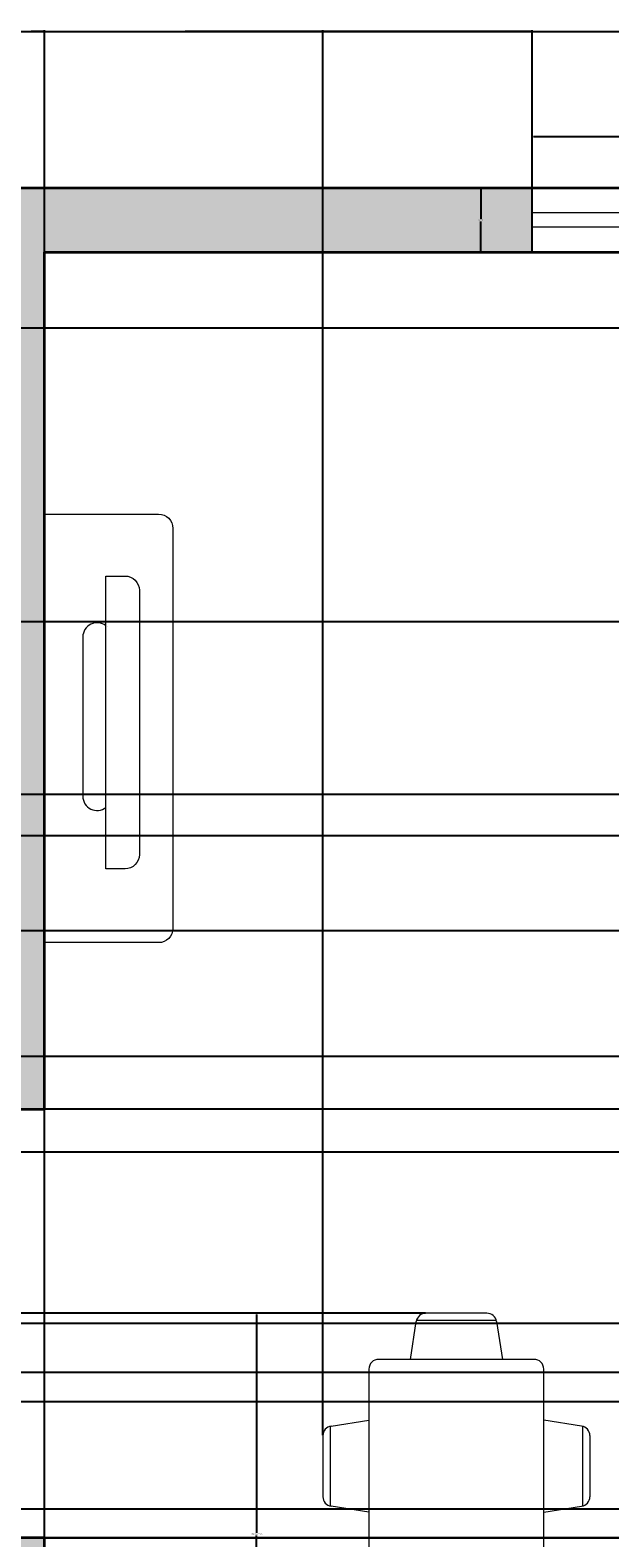
# Model space of a CAD drawing. Units: inches. Extents: x 2800 to 3283, y 1752 to 2114.
# Tile 4 of 6: x 2954 to 3035, y 1903 to 2114. Entities that reach past the tile are written whole.
import ezdxf

# ---------------------------------------------------------------- set-up
doc = ezdxf.new("R2010")
doc.units = ezdxf.units.IN
for name, color, linetype, lineweight in [('A-ANNO-DIMS', 2, 'Continuous', 18), ('A-FURN', 9, 'Continuous', 18), ('A-GLAZ', 4, 'Continuous', 18), ('A-WALL', 7, 'Continuous', 35)]:
    doc.layers.add(name, color=color, linetype=linetype, lineweight=lineweight)
doc.layers.add('A-WALL-PATT', color=18, linetype='Continuous', lineweight=13, true_color=0x000000)
doc.styles.get("Standard").update_dxf_attribs({"font": 'arial.ttf'})
doc.dimstyles.get("Standard").update_dxf_attribs({"dimtxt": 0.18, "dimasz": 0.18, "dimexe": 0.18, "dimexo": 0.0625, "dimgap": 0.09, "dimtad": 0, "dimtih": 1, "dimtoh": 1, "dimdec": 4, "dimzin": 0, "dimdsep": 46, "dimtxsty": 'Standard', "dimcen": 0.09, "dimadec": 0, "dimazin": 0, "dimtfac": 1, "dimtdec": 4, "dimtofl": 0, "dimtmove": 0, "dimatfit": 3, "dimfxl": 1, "dimtolj": 1, "dimtzin": 0, "dimarcsym": 0})

# ---------------------------------------------------------------- blocks, each defined once
blk = doc.blocks.new('Dining Set - 36 x 72 in.')
for p, q in [((-22.26, 25.81), (-23.48, 18)), ((-22.22, 26), (-5.78, 26)), ((-20.29, 27.5), (-7.71, 27.5)), ((-4.52, 18), (-5.74, 25.81)), ((5.74, 25.81), (4.52, 18)), ((5.78, 26), (22.22, 26)), ((7.71, 27.5), (20.29, 27.5)), ((23.48, 18), (22.26, 25.81)), ((-36, 16), (-36, -16)), ((34, 18), (-34, 18)), ((36, -16), (36, 16)), ((-43.81, 8.26), (-36, 9.48)), ((43.81, 8.26), (36, 9.48)), ((-45.5, 6.29), (-45.5, -6.29)), ((-44, 8.22), (-44, -8.22)), ((44, 8.22), (44, -8.22)), ((45.5, 6.29), (45.5, -6.29)), ((-36, -9.48), (-43.81, -8.26)), ((36, -9.48), (43.81, -8.26)), ((-34, -18), (34, -18)), ((-22.26, -25.81), (-23.48, -18)), ((-4.52, -18), (-5.74, -25.81)), ((5.74, -25.81), (4.52, -18)), ((23.48, -18), (22.26, -25.81)), ((-22.22, -26), (-5.78, -26)), ((-20.29, -27.5), (-7.71, -27.5)), ((5.78, -26), (22.22, -26)), ((7.71, -27.5), (20.29, -27.5))]:
    blk.add_line(p, q)
for centre, start, end in [((-20.29, 25.5), 90, 171.1198), ((-7.71, 25.5), 8.881, 90), ((7.71, 25.5), 90, 171.1198), ((20.29, 25.5), 8.881, 90), ((-34, 16), 90, 180), ((34, 16), 0, 90), ((-43.5, 6.29), 98.8806, 180), ((43.5, 6.29), 0, 81.1194), ((-43.5, -6.29), 180, 261.1194), ((43.5, -6.29), 278.8806, 0), ((-34, -16), 180, 270), ((34, -16), 270, 0), ((-20.29, -25.5), 188.8802, 270), ((-7.71, -25.5), 270, 351.1191), ((7.71, -25.5), 188.8802, 270), ((20.29, -25.5), 270, 351.1191)]:
    blk.add_arc(centre, 2, start, end)
blk = doc.blocks.new('WIN-48')
for p, q in [((0, 5.5), (48, 5.5)), ((0, 3.5), (48, 3.5))]:
    blk.add_line(p, q)
for points in [[(0, 0), (0, 9)], [(48, 9), (48, 0)]]:
    blk.add_lwpolyline(points)
blk = doc.blocks.new('MEDIA-CONSOLE-60')
for points in [[(0, 60), (16, 60, -0.414214), (18, 58), (18, 2, -0.414214), (16, 0), (0, 0)], [(8.61, 51.33), (11.3, 51.33, -0.414214), (13.3, 49.33), (13.3, 12.33, -0.414214), (11.3, 10.33), (8.61, 10.33)]]:
    blk.add_lwpolyline(points, format="xyb", close=True)
blk.add_lwpolyline([(8.61, 15.1), (8.61, 47.68)])
blk.add_lwpolyline([(8.61, 44.37, 0.62446), (5.38, 42.79), (5.38, 20.5, 0.62446), (8.61, 18.92, 0.62446)], format="xyb")
blk = doc.blocks.new('*D19')
at = {"layer": 'A-ANNO-DIMS', "color": 0, "lineweight": -2, "transparency": 16777216}
for p, q in [((3023.88, 2092.33), (3023.88, 2099.65)), ((3024.06, 2099.47), (3046.76, 2099.47)), ((3071.7, 2099.47), (3049, 2099.47)), ((3071.88, 2092.33), (3071.88, 2099.65))]:
    blk.add_line(p, q, dxfattribs=at)
at = {"layer": 'A-ANNO-DIMS', "color": 0, "transparency": 16777216}
for points in [[(3024.06, 2099.5), (3024.06, 2099.44), (3023.88, 2099.47)], [(3071.7, 2099.5), (3071.7, 2099.44), (3071.88, 2099.47)]]:
    blk.add_solid(points, dxfattribs=at)
at = {"layer": 'Defpoints', "color": 0, "transparency": 16777216}
for p in [(3023.88, 2099.47), (3023.88, 2092.27), (3071.88, 2092.27)]:
    blk.add_point(p, dxfattribs=at)
at = {"layer": 'A-ANNO-DIMS', "color": 0, "transparency": 16777216, "insert": (3047.88, 2099.47), "char_height": 0.18, "attachment_point": 5}
blk.add_mtext('\\A1;WINDOW 48 TYP.', dxfattribs=at)
blk = doc.blocks.new('*D20')
at = {"layer": 'A-ANNO-DIMS', "color": 0, "lineweight": -2, "transparency": 16777216}
for p, q in [((3023.82, 2092.27), (3016.5, 2092.27)), ((3016.68, 2092.09), (3016.68, 2087.95)), ((3016.68, 2083.45), (3016.68, 2087.59)), ((3023.82, 2083.27), (3016.5, 2083.27))]:
    blk.add_line(p, q, dxfattribs=at)
at = {"layer": 'A-ANNO-DIMS', "color": 0, "transparency": 16777216}
for points in [[(3016.65, 2092.09), (3016.71, 2092.09), (3016.68, 2092.27)], [(3016.65, 2083.45), (3016.71, 2083.45), (3016.68, 2083.27)]]:
    blk.add_solid(points, dxfattribs=at)
at = {"layer": 'Defpoints', "color": 0, "transparency": 16777216}
for p in [(3023.88, 2092.27), (3016.68, 2083.27), (3023.88, 2083.27)]:
    blk.add_point(p, dxfattribs=at)
at = {"layer": 'A-ANNO-DIMS', "color": 0, "transparency": 16777216, "insert": (3016.68, 2087.77), "char_height": 0.18, "attachment_point": 5}
blk.add_mtext('\\A1;9 TYP.', dxfattribs=at)
blk = doc.blocks.new('*D35')
at = {"layer": 'A-ANNO-DIMS', "color": 0, "lineweight": -2, "transparency": 16777216}
for p, q in [((2994.48, 1934.72), (2985.08, 1934.72)), ((2985.26, 1934.54), (2985.26, 1903.97)), ((2985.26, 1873.03), (2985.26, 1903.6)), ((2994.48, 1872.85), (2985.08, 1872.85))]:
    blk.add_line(p, q, dxfattribs=at)
at = {"layer": 'A-ANNO-DIMS', "color": 0, "transparency": 16777216}
for points in [[(2985.23, 1934.54), (2985.29, 1934.54), (2985.26, 1934.72)], [(2985.23, 1873.03), (2985.29, 1873.03), (2985.26, 1872.85)]]:
    blk.add_solid(points, dxfattribs=at)
at = {"layer": 'Defpoints', "color": 0, "transparency": 16777216}
for p in [(2994.54, 1934.72), (2985.26, 1872.85), (2994.54, 1872.85)]:
    blk.add_point(p, dxfattribs=at)
at = {"layer": 'A-ANNO-DIMS', "color": 0, "transparency": 16777216, "insert": (2985.26, 1903.79), "char_height": 0.18, "attachment_point": 5}
blk.add_mtext('\\A1;DINING SET 62', dxfattribs=at)
blk = doc.blocks.new('*D43')
at = {"layer": 'A-ANNO-DIMS', "color": 0, "lineweight": -2, "transparency": 16777216}
for p, q in [((2822.54, 2092.33), (2822.54, 2114.36)), ((2822.72, 2114.18), (3041.25, 2114.18)), ((3260.36, 2114.18), (3041.84, 2114.18)), ((3260.54, 2092.33), (3260.54, 2114.36))]:
    blk.add_line(p, q, dxfattribs=at)
at = {"layer": 'A-ANNO-DIMS', "color": 0, "transparency": 16777216}
for points in [[(2822.72, 2114.21), (2822.72, 2114.15), (2822.54, 2114.18)], [(3260.36, 2114.21), (3260.36, 2114.15), (3260.54, 2114.18)]]:
    blk.add_solid(points, dxfattribs=at)
at = {"layer": 'Defpoints', "color": 0, "transparency": 16777216}
for p in [(3260.54, 2114.18), (2822.54, 2092.27), (3260.54, 2092.27)]:
    blk.add_point(p, dxfattribs=at)
at = {"layer": 'A-ANNO-DIMS', "color": 0, "transparency": 16777216, "insert": (3041.54, 2114.18), "char_height": 0.18, "attachment_point": 5}
blk.add_mtext('\\A1;438', dxfattribs=at)
blk = doc.blocks.new('*D46')
at = {"layer": 'A-ANNO-DIMS', "color": 0, "lineweight": -2, "transparency": 16777216}
for p, q in [((2951.54, 2083.33), (2951.54, 2114.36)), ((2951.72, 2114.18), (2953.39, 2114.18)), ((2955.36, 2114.18), (2953.7, 2114.18)), ((2955.54, 2083.33), (2955.54, 2114.36))]:
    blk.add_line(p, q, dxfattribs=at)
at = {"layer": 'A-ANNO-DIMS', "color": 0, "transparency": 16777216}
for points in [[(2951.72, 2114.21), (2951.72, 2114.15), (2951.54, 2114.18)], [(2955.36, 2114.21), (2955.36, 2114.15), (2955.54, 2114.18)]]:
    blk.add_solid(points, dxfattribs=at)
at = {"layer": 'Defpoints', "color": 0, "transparency": 16777216}
for p in [(2955.54, 2114.18), (2951.54, 2083.27), (2955.54, 2083.27)]:
    blk.add_point(p, dxfattribs=at)
at = {"layer": 'A-ANNO-DIMS', "color": 0, "transparency": 16777216, "insert": (2953.54, 2114.18), "char_height": 0.18, "attachment_point": 5}
blk.add_mtext('\\A1;4', dxfattribs=at)
blk = doc.blocks.new('*D47')
at = {"layer": 'A-ANNO-DIMS', "color": 0, "lineweight": -2, "transparency": 16777216}
for p, q in [((2955.54, 1963.33), (2955.54, 2114.36)), ((2955.72, 2114.18), (3041.26, 2114.18)), ((3127.36, 2114.18), (3041.82, 2114.18)), ((3127.54, 1963.33), (3127.54, 2114.36))]:
    blk.add_line(p, q, dxfattribs=at)
at = {"layer": 'A-ANNO-DIMS', "color": 0, "transparency": 16777216}
for points in [[(2955.72, 2114.21), (2955.72, 2114.15), (2955.54, 2114.18)], [(3127.36, 2114.21), (3127.36, 2114.15), (3127.54, 2114.18)]]:
    blk.add_solid(points, dxfattribs=at)
at = {"layer": 'Defpoints', "color": 0, "transparency": 16777216}
for p in [(3127.54, 2114.18), (2955.54, 1963.27), (3127.54, 1963.27)]:
    blk.add_point(p, dxfattribs=at)
at = {"layer": 'A-ANNO-DIMS', "color": 0, "transparency": 16777216, "insert": (3041.54, 2114.18), "char_height": 0.18, "attachment_point": 5}
blk.add_mtext('\\A1;172', dxfattribs=at)
blk = doc.blocks.new('*D57')
at = {"layer": 'A-ANNO-DIMS', "color": 0, "lineweight": -2, "transparency": 16777216}
for p, q in [((2955.54, 2083.33), (2955.54, 2114.36)), ((2955.72, 2114.18), (2989.32, 2114.18)), ((3023.7, 2114.18), (2990.11, 2114.18)), ((3023.88, 2083.33), (3023.88, 2114.36))]:
    blk.add_line(p, q, dxfattribs=at)
at = {"layer": 'A-ANNO-DIMS', "color": 0, "transparency": 16777216}
for points in [[(2955.72, 2114.21), (2955.72, 2114.15), (2955.54, 2114.18)], [(3023.7, 2114.21), (3023.7, 2114.15), (3023.88, 2114.18)]]:
    blk.add_solid(points, dxfattribs=at)
at = {"layer": 'Defpoints', "color": 0, "transparency": 16777216}
for p in [(3023.88, 2114.18), (2955.54, 2083.27), (3023.88, 2083.27)]:
    blk.add_point(p, dxfattribs=at)
at = {"layer": 'A-ANNO-DIMS', "color": 0, "transparency": 16777216, "insert": (2989.71, 2114.18), "char_height": 0.18, "attachment_point": 5}
blk.add_mtext('\\A1;68.34', dxfattribs=at)
blk = doc.blocks.new('*D64')
at = {"layer": 'A-ANNO-DIMS', "color": 0, "lineweight": -2, "transparency": 16777216}
for p, q in [((2831.61, 1922.35), (3282.64, 1922.35)), ((3282.46, 1922.17), (3282.46, 1912.99)), ((3282.46, 1903.45), (3282.46, 1912.63)), ((2831.61, 1903.27), (3282.64, 1903.27))]:
    blk.add_line(p, q, dxfattribs=at)
at = {"layer": 'A-ANNO-DIMS', "color": 0, "transparency": 16777216}
for points in [[(3282.43, 1922.17), (3282.49, 1922.17), (3282.46, 1922.35)], [(3282.43, 1903.45), (3282.49, 1903.45), (3282.46, 1903.27)]]:
    blk.add_solid(points, dxfattribs=at)
at = {"layer": 'Defpoints', "color": 0, "transparency": 16777216}
for p in [(2831.54, 1922.35), (3282.46, 1922.35), (2831.54, 1903.27)]:
    blk.add_point(p, dxfattribs=at)
at = {"layer": 'A-ANNO-DIMS', "color": 0, "transparency": 16777216, "insert": (3282.46, 1912.81), "char_height": 0.18, "attachment_point": 5}
blk.add_mtext('\\A1;19.085', dxfattribs=at)
blk = doc.blocks.new('*D65')
at = {"layer": 'A-ANNO-DIMS', "color": 0, "lineweight": -2, "transparency": 16777216}
for p, q in [((3251.48, 1926.4), (2800.45, 1926.4)), ((2800.63, 1926.22), (2800.63, 1917.02)), ((2800.63, 1907.45), (2800.63, 1916.65)), ((3251.48, 1907.27), (2800.45, 1907.27))]:
    blk.add_line(p, q, dxfattribs=at)
at = {"layer": 'A-ANNO-DIMS', "color": 0, "transparency": 16777216}
for points in [[(2800.6, 1926.22), (2800.66, 1926.22), (2800.63, 1926.4)], [(2800.6, 1907.45), (2800.66, 1907.45), (2800.63, 1907.27)]]:
    blk.add_solid(points, dxfattribs=at)
at = {"layer": 'Defpoints', "color": 0, "transparency": 16777216}
for p in [(2800.63, 1926.4), (3251.54, 1926.4), (3251.54, 1907.27)]:
    blk.add_point(p, dxfattribs=at)
at = {"layer": 'A-ANNO-DIMS', "color": 0, "transparency": 16777216, "insert": (2800.63, 1916.83), "char_height": 0.18, "attachment_point": 5}
blk.add_mtext('\\A1;19.128', dxfattribs=at)
blk = doc.blocks.new('*D68')
at = {"layer": 'A-ANNO-DIMS', "color": 0, "lineweight": -2, "transparency": 16777216}
for p, q in [((3175.48, 1957.27), (2800.45, 1957.27)), ((2800.63, 1957.09), (2800.63, 1945.45)), ((2800.63, 1933.45), (2800.63, 1945.09)), ((3175.48, 1933.27), (2800.45, 1933.27))]:
    blk.add_line(p, q, dxfattribs=at)
at = {"layer": 'A-ANNO-DIMS', "color": 0, "transparency": 16777216}
for points in [[(2800.6, 1957.09), (2800.66, 1957.09), (2800.63, 1957.27)], [(2800.6, 1933.45), (2800.66, 1933.45), (2800.63, 1933.27)]]:
    blk.add_solid(points, dxfattribs=at)
at = {"layer": 'Defpoints', "color": 0, "transparency": 16777216}
for p in [(2800.63, 1957.27), (3175.54, 1957.27), (3175.54, 1933.27)]:
    blk.add_point(p, dxfattribs=at)
at = {"layer": 'A-ANNO-DIMS', "color": 0, "transparency": 16777216, "insert": (2800.63, 1945.27), "char_height": 0.18, "attachment_point": 5}
blk.add_mtext('\\A1;24', dxfattribs=at)
blk = doc.blocks.new('*D69')
at = {"layer": 'A-ANNO-DIMS', "color": 0, "lineweight": -2, "transparency": 16777216}
for p, q in [((3175.48, 1963.27), (2800.45, 1963.27)), ((2800.63, 1963.09), (2800.63, 1960.45)), ((2800.63, 1957.45), (2800.63, 1960.09)), ((3175.48, 1957.27), (2800.45, 1957.27))]:
    blk.add_line(p, q, dxfattribs=at)
at = {"layer": 'A-ANNO-DIMS', "color": 0, "transparency": 16777216}
for points in [[(2800.6, 1963.09), (2800.66, 1963.09), (2800.63, 1963.27)], [(2800.6, 1957.45), (2800.66, 1957.45), (2800.63, 1957.27)]]:
    blk.add_solid(points, dxfattribs=at)
at = {"layer": 'Defpoints', "color": 0, "transparency": 16777216}
for p in [(2800.63, 1963.27), (3175.54, 1963.27), (3175.54, 1957.27)]:
    blk.add_point(p, dxfattribs=at)
at = {"layer": 'A-ANNO-DIMS', "color": 0, "transparency": 16777216, "insert": (2800.63, 1960.27), "char_height": 0.18, "attachment_point": 5}
blk.add_mtext('\\A1;6', dxfattribs=at)
blk = doc.blocks.new('*D71')
at = {"layer": 'A-ANNO-DIMS', "color": 0, "lineweight": -2, "transparency": 16777216}
for p, q in [((3037.48, 1903.27), (2800.45, 1903.27)), ((2800.63, 1903.09), (2800.63, 1879.54)), ((2800.63, 1855.63), (2800.63, 1879.18)), ((3037.48, 1855.45), (2800.45, 1855.45))]:
    blk.add_line(p, q, dxfattribs=at)
at = {"layer": 'A-ANNO-DIMS', "color": 0, "transparency": 16777216}
for points in [[(2800.6, 1903.09), (2800.66, 1903.09), (2800.63, 1903.27)], [(2800.6, 1855.63), (2800.66, 1855.63), (2800.63, 1855.45)]]:
    blk.add_solid(points, dxfattribs=at)
at = {"layer": 'Defpoints', "color": 0, "transparency": 16777216}
for p in [(2800.63, 1903.27), (3037.54, 1903.27), (3037.54, 1855.45)]:
    blk.add_point(p, dxfattribs=at)
at = {"layer": 'A-ANNO-DIMS', "color": 0, "transparency": 16777216, "insert": (2800.63, 1879.36), "char_height": 0.18, "attachment_point": 5}
blk.add_mtext('\\A1;47.82', dxfattribs=at)
blk = doc.blocks.new('*D76')
at = {"layer": 'A-ANNO-DIMS', "color": 0, "lineweight": -2, "transparency": 16777216}
for p, q in [((3095.48, 1903.27), (2800.45, 1903.27)), ((2800.63, 1903.09), (2800.63, 1891.49)), ((2800.63, 1879.52), (2800.63, 1891.12)), ((3103.48, 1879.34), (2800.45, 1879.34))]:
    blk.add_line(p, q, dxfattribs=at)
at = {"layer": 'A-ANNO-DIMS', "color": 0, "transparency": 16777216}
for points in [[(2800.6, 1903.09), (2800.66, 1903.09), (2800.63, 1903.27)], [(2800.6, 1879.52), (2800.66, 1879.52), (2800.63, 1879.34)]]:
    blk.add_solid(points, dxfattribs=at)
at = {"layer": 'Defpoints', "color": 0, "transparency": 16777216}
for p in [(3095.54, 1903.27), (2800.63, 1879.34), (3103.54, 1879.34)]:
    blk.add_point(p, dxfattribs=at)
at = {"layer": 'A-ANNO-DIMS', "color": 0, "transparency": 16777216, "insert": (2800.63, 1891.31), "char_height": 0.18, "attachment_point": 5}
blk.add_mtext('\\A1;23.93', dxfattribs=at)
blk = doc.blocks.new('*D77')
at = {"layer": 'A-ANNO-DIMS', "color": 0, "lineweight": -2, "transparency": 16777216}
for p, q in [((3076.62, 2072.66), (2800.45, 2072.66)), ((2800.63, 2072.48), (2800.63, 2021.84)), ((2800.63, 1970.84), (2800.63, 2021.48)), ((3076.62, 1970.66), (2800.45, 1970.66))]:
    blk.add_line(p, q, dxfattribs=at)
at = {"layer": 'A-ANNO-DIMS', "color": 0, "transparency": 16777216}
for points in [[(2800.6, 2072.48), (2800.66, 2072.48), (2800.63, 2072.66)], [(2800.6, 1970.84), (2800.66, 1970.84), (2800.63, 1970.66)]]:
    blk.add_solid(points, dxfattribs=at)
at = {"layer": 'Defpoints', "color": 0, "transparency": 16777216}
for p in [(3076.68, 2072.66), (2800.63, 1970.66), (3076.68, 1970.66)]:
    blk.add_point(p, dxfattribs=at)
at = {"layer": 'A-ANNO-DIMS', "color": 0, "transparency": 16777216, "insert": (2800.63, 2021.66), "char_height": 0.18, "attachment_point": 5}
blk.add_mtext('\\A1;102', dxfattribs=at)
blk = doc.blocks.new('*D80')
at = {"layer": 'A-ANNO-DIMS', "color": 0, "lineweight": -2, "transparency": 16777216}
for p, q in [((3045.08, 2031.54), (2800.45, 2031.54)), ((2800.63, 2031.36), (2800.63, 2016.73)), ((2800.63, 2001.72), (2800.63, 2016.36)), ((3045.08, 2001.54), (2800.45, 2001.54))]:
    blk.add_line(p, q, dxfattribs=at)
at = {"layer": 'A-ANNO-DIMS', "color": 0, "transparency": 16777216}
for points in [[(2800.6, 2031.36), (2800.66, 2031.36), (2800.63, 2031.54)], [(2800.6, 2001.72), (2800.66, 2001.72), (2800.63, 2001.54)]]:
    blk.add_solid(points, dxfattribs=at)
at = {"layer": 'Defpoints', "color": 0, "transparency": 16777216}
for p in [(2800.63, 2031.54), (3045.14, 2031.54), (3045.14, 2001.54)]:
    blk.add_point(p, dxfattribs=at)
at = {"layer": 'A-ANNO-DIMS', "color": 0, "transparency": 16777216, "insert": (2800.63, 2016.54), "char_height": 0.18, "attachment_point": 5}
blk.add_mtext('\\A1;30', dxfattribs=at)
blk = doc.blocks.new('*D82')
at = {"layer": 'A-ANNO-DIMS', "color": 0, "lineweight": -2, "transparency": 16777216}
for p, q in [((3171.82, 2007.36), (2800.45, 2007.36)), ((2800.63, 2007.18), (2800.63, 1998)), ((2800.63, 1988.45), (2800.63, 1997.63)), ((3179.48, 1988.27), (2800.45, 1988.27))]:
    blk.add_line(p, q, dxfattribs=at)
at = {"layer": 'A-ANNO-DIMS', "color": 0, "transparency": 16777216}
for points in [[(2800.6, 2007.18), (2800.66, 2007.18), (2800.63, 2007.36)], [(2800.6, 1988.45), (2800.66, 1988.45), (2800.63, 1988.27)]]:
    blk.add_solid(points, dxfattribs=at)
at = {"layer": 'Defpoints', "color": 0, "transparency": 16777216}
for p in [(2800.63, 2007.36), (3171.89, 2007.36), (3179.54, 1988.27)]:
    blk.add_point(p, dxfattribs=at)
at = {"layer": 'A-ANNO-DIMS', "color": 0, "transparency": 16777216, "insert": (2800.63, 1997.81), "char_height": 0.18, "attachment_point": 5}
blk.add_mtext('\\A1;19.09', dxfattribs=at)
blk = doc.blocks.new('*D85')
at = {"layer": 'A-ANNO-DIMS', "color": 0, "lineweight": -2, "transparency": 16777216}
for p, q in [((2955.54, 1903.33), (2955.54, 2114.36)), ((2955.72, 2114.18), (2974.82, 2114.18)), ((2994.36, 2114.18), (2975.26, 2114.18)), ((2994.54, 1917.64), (2994.54, 2114.36))]:
    blk.add_line(p, q, dxfattribs=at)
at = {"layer": 'A-ANNO-DIMS', "color": 0, "transparency": 16777216}
for points in [[(2955.72, 2114.21), (2955.72, 2114.15), (2955.54, 2114.18)], [(2994.36, 2114.21), (2994.36, 2114.15), (2994.54, 2114.18)]]:
    blk.add_solid(points, dxfattribs=at)
at = {"layer": 'Defpoints', "color": 0, "transparency": 16777216}
for p in [(2994.54, 2114.18), (2994.54, 1917.58), (2955.54, 1903.27)]:
    blk.add_point(p, dxfattribs=at)
at = {"layer": 'A-ANNO-DIMS', "color": 0, "transparency": 16777216, "insert": (2975.04, 2114.18), "char_height": 0.18, "attachment_point": 5}
blk.add_mtext('\\A1;39', dxfattribs=at)
blk = doc.blocks.new('*D86')
at = {"layer": 'A-ANNO-DIMS', "color": 0, "lineweight": -2, "transparency": 16777216}
for p, q in [((2955.48, 1963.27), (2800.45, 1963.27)), ((2800.63, 1963.09), (2800.63, 1949.18)), ((2800.63, 1934.9), (2800.63, 1948.81)), ((3008.9, 1934.72), (2800.45, 1934.72))]:
    blk.add_line(p, q, dxfattribs=at)
at = {"layer": 'A-ANNO-DIMS', "color": 0, "transparency": 16777216}
for points in [[(2800.6, 1963.09), (2800.66, 1963.09), (2800.63, 1963.27)], [(2800.6, 1934.9), (2800.66, 1934.9), (2800.63, 1934.72)]]:
    blk.add_solid(points, dxfattribs=at)
at = {"layer": 'Defpoints', "color": 0, "transparency": 16777216}
for p in [(2955.54, 1963.27), (2800.63, 1934.72), (3008.97, 1934.72)]:
    blk.add_point(p, dxfattribs=at)
at = {"layer": 'A-ANNO-DIMS', "color": 0, "transparency": 16777216, "insert": (2800.63, 1949), "char_height": 0.18, "attachment_point": 5}
blk.add_mtext('\\A1;28.547', dxfattribs=at)

msp = doc.modelspace()

# ---------------------------------------------------------------- hatches: boundary and pattern name
at = {"layer": 'A-WALL-PATT'}
h = msp.add_hatch(color=256, dxfattribs=at)
h.dxf.hatch_style = 1
h.paths.add_polyline_path([(3023.883, 2092.2695), (2916.6629, 2092.2695), (2916.6629, 2083.2695), (2951.5432, 2083.2695), (2951.5432, 2011.2695), (2951.5432, 1967.2695), (2945.5432, 1967.2695), (2945.5432, 1963.2695), (2955.5432, 1963.2695), (2955.5432, 2083.2695), (3023.883, 2083.2695)])
h = msp.add_hatch(color=256, dxfattribs=at)
h.dxf.hatch_style = 1
h.paths.add_polyline_path([(2967.5432, 1783.2695), (2955.5432, 1783.2695), (2955.5432, 1903.2695), (2945.5432, 1903.2695), (2945.5432, 1899.2695), (2951.5432, 1899.2695), (2951.5432, 1783.2695), (2911.5307, 1783.2695), (2911.5307, 1774.2695), (2967.5432, 1774.2695)])

# ---------------------------------------------------------------- linework, layer by layer
at = {"layer": 'A-FURN'}
msp.add_lwpolyline([(2964.3483, 2030.799), (2964.3483, 2030.799)], close=True, dxfattribs=at)
at = {"layer": 'A-WALL'}
for p, q in [((2955.5432, 2083.2695), (3127.5432, 2083.2695)), ((2955.5432, 1963.2695), (2955.5432, 2083.2695)), ((2945.5432, 1963.2695), (2955.5432, 1963.2695)), ((2955.5432, 1903.2695), (2945.5432, 1903.2695)), ((2955.5432, 1783.2695), (2955.5432, 1903.2695))]:
    msp.add_line(p, q, dxfattribs=at)
msp.add_lwpolyline([(2967.5432, 1774.2695), (2822.5432, 1774.2695), (2822.5432, 2092.2695), (3260.5432, 2092.2695), (3260.5432, 1774.2695), (3015.5432, 1774.2695)], dxfattribs=at)

# ---------------------------------------------------------------- block references
at = {"layer": 'A-FURN'}
msp.add_blockref('MEDIA-CONSOLE-60', (2955.543, 1986.609), dxfattribs=at)
at = {"layer": 'A-FURN', "xscale": 0.6798973634336658, "yscale": 0.6798973634336658, "zscale": 0.6798973634336658, "rotation": 270}
msp.add_blockref('Dining Set - 36 x 72 in.', (3013.2412, 1903.787), dxfattribs=at)
at = {"layer": 'A-GLAZ', "rotation": 180}
msp.add_blockref('WIN-48', (3071.8829, 2092.269), dxfattribs=at)

# ---------------------------------------------------------------- dimensions: what is measured, and where the dimension line sits
at = {"layer": 'A-ANNO-DIMS'}
for base, p1, p2, override, picture, middle in [((3260.5432, 2114.1845), (2822.5432, 2092.2695), (3260.5432, 2092.2695), {"dimdec": 0, "dimlfac": 1, "dimrnd": 0, "dimzin": 0, "dimdsep": 46, "dimlunit": 2}, '*D43', (3041.5432, 2114.1845)), ((2955.5432, 2114.1845), (2951.5432, 2083.2695), (2955.5432, 2083.2695), {"dimdec": 0, "dimlfac": 1, "dimrnd": 0, "dimzin": 0, "dimdsep": 46, "dimlunit": 2}, '*D46', (2953.5432, 2114.1845)), ((3127.5432, 2114.1845), (2955.5432, 1963.2695), (3127.5432, 1963.2695), {"dimdec": 0, "dimlfac": 1, "dimrnd": 0, "dimzin": 0, "dimdsep": 46, "dimlunit": 2}, '*D47', (3041.5432, 2114.1845)), ((3023.883, 2114.1845), (2955.5432, 2083.2695), (3023.883, 2083.2695), {"dimdec": 2, "dimlfac": 1, "dimrnd": 0, "dimzin": 0, "dimdsep": 46, "dimlunit": 2}, '*D57', (2989.7131, 2114.1845)), ((2994.5441, 2114.1845), (2955.5432, 1903.2695), (2994.5441, 1917.581), {"dimdec": 0, "dimlfac": 1, "dimrnd": 0, "dimzin": 0, "dimdsep": 46, "dimlunit": 2}, '*D85', (2975.0436, 2114.1845))]:
    dim = msp.add_linear_dim(base=base, p1=p1, p2=p2, dimstyle='Standard', override=override, dxfattribs=at)
    dim.commit()
    dim.dimension.update_dxf_attribs({"geometry": picture, "text_midpoint": middle})
for base, p1, p2, angle, text, picture, middle in [((3023.883, 2099.4695), (3071.883, 2092.2695), (3023.883, 2092.2695), 180, 'WINDOW <> TYP.', '*D19', (3047.883, 2099.4695)), ((3016.683, 2083.2695), (3023.883, 2092.2695), (3023.883, 2083.2695), 270, '<> TYP.', '*D20', (3016.683, 2087.7695)), ((2985.2635, 1872.8517), (2994.5441, 1934.7224), (2994.5441, 1872.8517), 270, 'DINING SET <>', '*D35', (2985.2635, 1903.787))]:
    dim = msp.add_linear_dim(base=base, p1=p1, p2=p2, angle=angle, text=text, dimstyle='Standard', override={"dimdec": 0, "dimlfac": 1, "dimrnd": 0, "dimzin": 0, "dimdsep": 46, "dimlunit": 2}, dxfattribs=at)
    dim.commit()
    dim.dimension.update_dxf_attribs({"geometry": picture, "text_midpoint": middle})
for base, p1, p2, override, picture, middle in [((2800.6282, 1970.661), (3076.6778, 2072.661), (3076.6778, 1970.661), {"dimdec": 0, "dimlfac": 1, "dimrnd": 0, "dimzin": 0, "dimdsep": 46, "dimlunit": 2}, '*D77', (2800.6282, 2021.661)), ((2800.6282, 2031.544), (3045.1406, 2001.544), (3045.1406, 2031.544), {"dimdec": 0, "dimlfac": 1, "dimrnd": 0, "dimzin": 0, "dimdsep": 46, "dimlunit": 2}, '*D80', (2800.6282, 2016.544)), ((2800.6282, 2007.3598), (3179.5432, 1988.2695), (3171.8868, 2007.3598), {"dimdec": 2, "dimlfac": 1, "dimrnd": 0, "dimzin": 0, "dimdsep": 46, "dimlunit": 2}, '*D82', (2800.6282, 1997.8147)), ((2800.6282, 1934.7224), (2955.5432, 1963.2695), (3008.9659, 1934.7224), {"dimdec": 3, "dimlfac": 1, "dimrnd": 0, "dimzin": 0, "dimdsep": 46, "dimlunit": 2}, '*D86', (2800.6282, 1948.9959)), ((2800.6282, 1963.2695), (3175.5432, 1957.2695), (3175.5432, 1963.2695), {"dimdec": 0, "dimlfac": 1, "dimrnd": 0, "dimzin": 0, "dimdsep": 46, "dimlunit": 2}, '*D69', (2800.6282, 1960.2695)), ((2800.6282, 1957.2695), (3175.5432, 1933.2695), (3175.5432, 1957.2695), {"dimdec": 0, "dimlfac": 1, "dimrnd": 0, "dimzin": 0, "dimdsep": 46, "dimlunit": 2}, '*D68', (2800.6282, 1945.2695)), ((2800.6282, 1926.3971), (3251.5432, 1907.2695), (3251.5432, 1926.3971), {"dimdec": 3, "dimlfac": 1, "dimrnd": 0, "dimzin": 0, "dimdsep": 46, "dimlunit": 2}, '*D65', (2800.6282, 1916.8333)), ((3282.4582, 1922.3547), (2831.5432, 1903.2695), (2831.5432, 1922.3547), {"dimdec": 3, "dimlfac": 1, "dimrnd": 0, "dimzin": 0, "dimdsep": 46, "dimlunit": 2}, '*D64', (3282.4582, 1912.8121)), ((2800.6282, 1903.2695), (3037.5432, 1855.4517), (3037.5432, 1903.2695), {"dimdec": 2, "dimlfac": 1, "dimrnd": 0, "dimzin": 0, "dimdsep": 46, "dimlunit": 2}, '*D71', (2800.6282, 1879.3606)), ((2800.6282, 1879.3408), (3095.5432, 1903.2695), (3103.5432, 1879.3408), {"dimdec": 2, "dimlfac": 1, "dimrnd": 0, "dimzin": 0, "dimdsep": 46, "dimlunit": 2}, '*D76', (2800.6282, 1891.3052))]:
    dim = msp.add_linear_dim(base=base, p1=p1, p2=p2, angle=90, dimstyle='Standard', override=override, dxfattribs=at)
    dim.commit()
    dim.dimension.update_dxf_attribs({"geometry": picture, "text_midpoint": middle})

doc.saveas('drawing.dxf')
